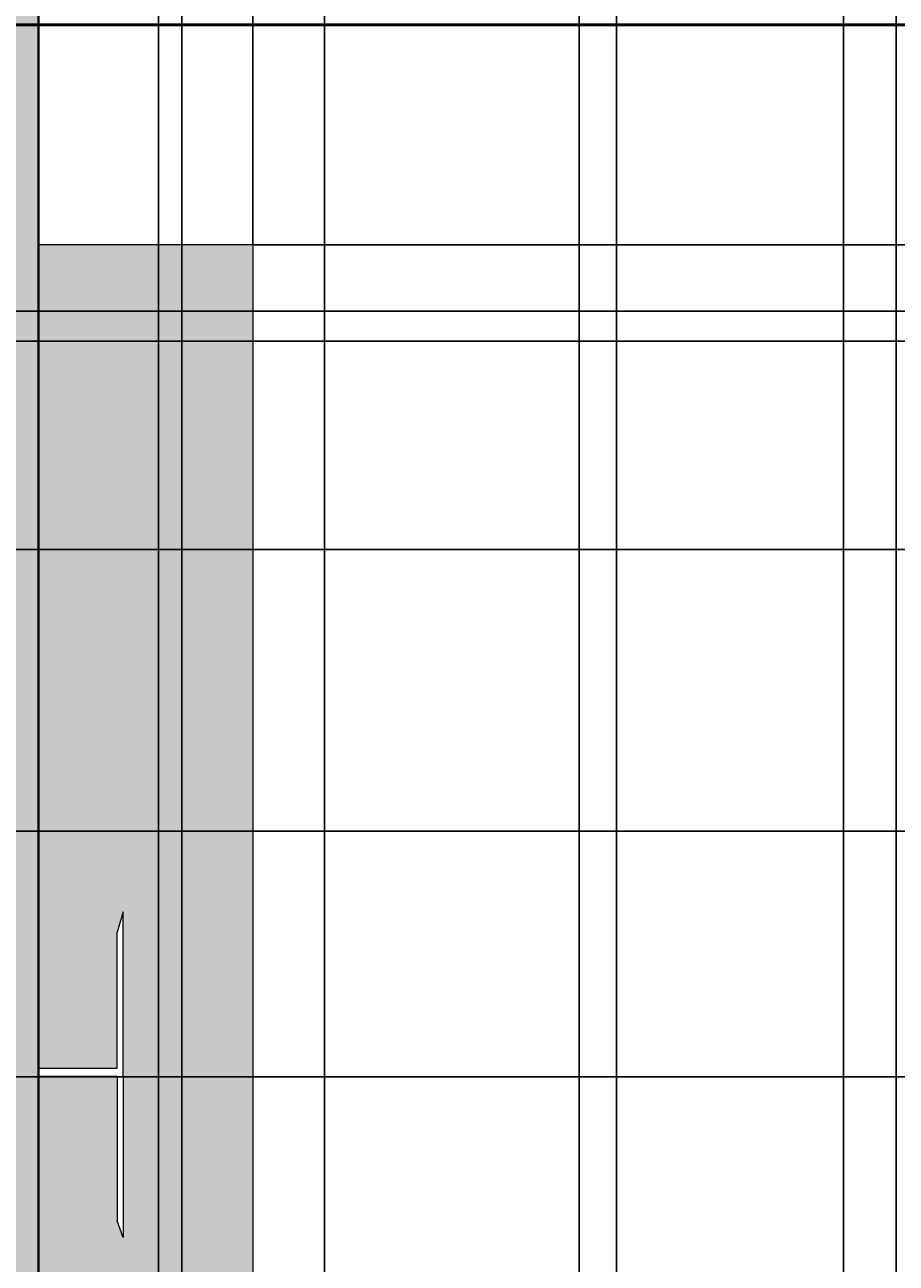
# Model space of a CAD drawing. Units: inches. Extents: x 818 to 1898, y 976 to 2364.
# Tile 26 of 96: x 1439 to 1512, y 1441 to 1545. Entities that reach past the tile are written whole.
import ezdxf

# ---------------------------------------------------------------- set-up
doc = ezdxf.new("R2010")
doc.units = ezdxf.units.IN
doc.header["$LTSCALE"] = 5
doc.header["$MEASUREMENT"] = 0
for name, color, linetype, lineweight in [('A-ANNO-DIMS', 2, 'Continuous', 18), ('A-EQPM', 8, 'Continuous', 18), ('A-FLOR-CASE', 8, 'Continuous', 18), ('A-FLOR-CASE-PATT', 33, 'Continuous', 9), ('A-WALL', 7, 'Continuous', 40)]:
    doc.layers.add(name, color=color, linetype=linetype, lineweight=lineweight)
doc.layers.add('A-WALL-PATT', color=251, linetype='Continuous', lineweight=13, true_color=0x636466)
doc.styles.get("Standard").update_dxf_attribs({"font": 'arial.ttf'})
doc.dimstyles.get("Standard").update_dxf_attribs({"dimtxt": 0.18, "dimasz": 0.18, "dimexe": 0.18, "dimexo": 0.0625, "dimgap": 0.09, "dimtad": 0, "dimtih": 1, "dimtoh": 1, "dimdec": 4, "dimzin": 0, "dimdsep": 46, "dimtxsty": 'Standard', "dimcen": 0.09, "dimadec": 0, "dimazin": 0, "dimtfac": 1, "dimtdec": 4, "dimtofl": 0, "dimtmove": 0, "dimatfit": 3, "dimfxl": 1, "dimtolj": 1, "dimtzin": 0, "dimarcsym": 0})

# ---------------------------------------------------------------- blocks, each defined once
blk = doc.blocks.new('*D99')
at = {"layer": 'A-ANNO-DIMS', "color": 0, "lineweight": -2, "ltscale": 5, "transparency": 16777216}
for p, q in [((1391.88, 1071.12), (1391.88, 2363.87)), ((1392.06, 2363.69), (1420.45, 2363.69)), ((1449.64, 2363.69), (1421.24, 2363.69)), ((1449.82, 1071.12), (1449.82, 2363.87))]:
    blk.add_line(p, q, dxfattribs=at)
at = {"layer": 'A-ANNO-DIMS', "color": 0, "ltscale": 5, "transparency": 16777216}
for points in [[(1392.06, 2363.72), (1392.06, 2363.66), (1391.88, 2363.69)], [(1449.64, 2363.72), (1449.64, 2363.66), (1449.82, 2363.69)]]:
    blk.add_solid(points, dxfattribs=at)
at = {"layer": 'Defpoints', "color": 0, "ltscale": 5, "transparency": 16777216}
for p in [(1449.82, 2363.69), (1391.88, 1071.06), (1449.82, 1071.06)]:
    blk.add_point(p, dxfattribs=at)
at = {"layer": 'A-ANNO-DIMS', "color": 0, "ltscale": 5, "transparency": 16777216, "insert": (1420.85, 2363.69), "char_height": 0.18, "attachment_point": 5}
blk.add_mtext('\\A1;57.94', dxfattribs=at)
blk = doc.blocks.new('*D100')
at = {"layer": 'A-ANNO-DIMS', "color": 0, "lineweight": -2, "ltscale": 5, "transparency": 16777216}
for p, q in [((1449.82, 1071.12), (1449.82, 2363.87)), ((1450, 2363.69), (1478.17, 2363.69)), ((1507.12, 2363.69), (1478.95, 2363.69)), ((1507.3, 1071.12), (1507.3, 2363.87))]:
    blk.add_line(p, q, dxfattribs=at)
at = {"layer": 'A-ANNO-DIMS', "color": 0, "ltscale": 5, "transparency": 16777216}
for points in [[(1450, 2363.72), (1450, 2363.66), (1449.82, 2363.69)], [(1507.12, 2363.72), (1507.12, 2363.66), (1507.3, 2363.69)]]:
    blk.add_solid(points, dxfattribs=at)
at = {"layer": 'Defpoints', "color": 0, "ltscale": 5, "transparency": 16777216}
for p in [(1507.3, 2363.69), (1449.82, 1071.06), (1507.3, 1071.06)]:
    blk.add_point(p, dxfattribs=at)
at = {"layer": 'A-ANNO-DIMS', "color": 0, "ltscale": 5, "transparency": 16777216, "insert": (1478.56, 2363.69), "char_height": 0.18, "attachment_point": 5}
blk.add_mtext('\\A1;57.48', dxfattribs=at)
blk = doc.blocks.new('*D101')
at = {"layer": 'A-ANNO-DIMS', "color": 0, "lineweight": -2, "ltscale": 5, "transparency": 16777216}
for p, q in [((1507.3, 1071.12), (1507.3, 2363.87)), ((1507.48, 2363.69), (1536, 2363.69)), ((1565.3, 2363.69), (1536.78, 2363.69)), ((1565.48, 1071.12), (1565.48, 2363.87))]:
    blk.add_line(p, q, dxfattribs=at)
at = {"layer": 'A-ANNO-DIMS', "color": 0, "ltscale": 5, "transparency": 16777216}
for points in [[(1507.48, 2363.72), (1507.48, 2363.66), (1507.3, 2363.69)], [(1565.3, 2363.72), (1565.3, 2363.66), (1565.48, 2363.69)]]:
    blk.add_solid(points, dxfattribs=at)
at = {"layer": 'Defpoints', "color": 0, "ltscale": 5, "transparency": 16777216}
for p in [(1565.48, 2363.69), (1507.3, 1071.06), (1565.48, 1071.06)]:
    blk.add_point(p, dxfattribs=at)
at = {"layer": 'A-ANNO-DIMS', "color": 0, "ltscale": 5, "transparency": 16777216, "insert": (1536.39, 2363.69), "char_height": 0.18, "attachment_point": 5}
blk.add_mtext('\\A1;58.19', dxfattribs=at)
blk = doc.blocks.new('*D116')
at = {"layer": 'A-ANNO-DIMS', "color": 0, "lineweight": -2, "ltscale": 5, "transparency": 16777216}
for p, q in [((1766.29, 1456.81), (818.03, 1456.81)), ((818.21, 1456.63), (818.21, 1417.41)), ((818.21, 1377.84), (818.21, 1417.05)), ((1766.29, 1377.66), (818.03, 1377.66))]:
    blk.add_line(p, q, dxfattribs=at)
at = {"layer": 'A-ANNO-DIMS', "color": 0, "ltscale": 5, "transparency": 16777216}
for points in [[(818.18, 1456.63), (818.24, 1456.63), (818.21, 1456.81)], [(818.18, 1377.84), (818.24, 1377.84), (818.21, 1377.66)]]:
    blk.add_solid(points, dxfattribs=at)
at = {"layer": 'Defpoints', "color": 0, "ltscale": 5, "transparency": 16777216}
for p in [(818.21, 1456.81), (1766.35, 1456.81), (1766.35, 1377.66)]:
    blk.add_point(p, dxfattribs=at)
at = {"layer": 'A-ANNO-DIMS', "color": 0, "ltscale": 5, "transparency": 16777216, "insert": (818.21, 1417.23), "char_height": 0.18, "attachment_point": 5}
blk.add_mtext('\\A1;79.15', dxfattribs=at)
blk = doc.blocks.new('*D117')
at = {"layer": 'A-ANNO-DIMS', "color": 0, "lineweight": -2, "ltscale": 5, "transparency": 16777216}
for p, q in [((1766.29, 1545.18), (818.03, 1545.18)), ((818.21, 1545), (818.21, 1501.18)), ((818.21, 1456.99), (818.21, 1500.81)), ((1766.29, 1456.81), (818.03, 1456.81))]:
    blk.add_line(p, q, dxfattribs=at)
at = {"layer": 'A-ANNO-DIMS', "color": 0, "ltscale": 5, "transparency": 16777216}
for points in [[(818.18, 1545), (818.24, 1545), (818.21, 1545.18)], [(818.18, 1456.99), (818.24, 1456.99), (818.21, 1456.81)]]:
    blk.add_solid(points, dxfattribs=at)
at = {"layer": 'Defpoints', "color": 0, "ltscale": 5, "transparency": 16777216}
for p in [(818.21, 1545.18), (1766.35, 1545.18), (1766.35, 1456.81)]:
    blk.add_point(p, dxfattribs=at)
at = {"layer": 'A-ANNO-DIMS', "color": 0, "ltscale": 5, "transparency": 16777216, "insert": (818.21, 1501), "char_height": 0.18, "attachment_point": 5}
blk.add_mtext('\\A1;88.37', dxfattribs=at)
blk = doc.blocks.new('*D159')
at = {"layer": 'A-ANNO-DIMS', "color": 0, "lineweight": -2, "ltscale": 5, "transparency": 16777216}
for p, q in [((1206.73, 1687.02), (1206.73, 975.66)), ((1463.73, 1687.02), (1463.73, 975.66)), ((1206.91, 975.84), (1334.93, 975.84)), ((1463.55, 975.84), (1335.52, 975.84))]:
    blk.add_line(p, q, dxfattribs=at)
at = {"layer": 'A-ANNO-DIMS', "color": 0, "ltscale": 5, "transparency": 16777216}
for points in [[(1206.91, 975.87), (1206.91, 975.81), (1206.73, 975.84)], [(1463.55, 975.87), (1463.55, 975.81), (1463.73, 975.84)]]:
    blk.add_solid(points, dxfattribs=at)
at = {"layer": 'Defpoints', "color": 0, "ltscale": 5, "transparency": 16777216}
for p in [(1206.73, 1687.08), (1463.73, 1687.08), (1463.73, 975.84)]:
    blk.add_point(p, dxfattribs=at)
at = {"layer": 'A-ANNO-DIMS', "color": 0, "ltscale": 5, "transparency": 16777216, "insert": (1335.23, 975.84), "char_height": 0.18, "attachment_point": 5}
blk.add_mtext('\\A1;257', dxfattribs=at)
blk = doc.blocks.new('*D160')
at = {"layer": 'A-ANNO-DIMS', "color": 0, "lineweight": -2, "ltscale": 5, "transparency": 16777216}
for p, q in [((1463.73, 1687.02), (1463.73, 975.66)), ((1511.73, 1687.02), (1511.73, 975.66)), ((1463.91, 975.84), (1487.5, 975.84)), ((1511.55, 975.84), (1487.95, 975.84))]:
    blk.add_line(p, q, dxfattribs=at)
at = {"layer": 'A-ANNO-DIMS', "color": 0, "ltscale": 5, "transparency": 16777216}
for points in [[(1463.91, 975.87), (1463.91, 975.81), (1463.73, 975.84)], [(1511.55, 975.87), (1511.55, 975.81), (1511.73, 975.84)]]:
    blk.add_solid(points, dxfattribs=at)
at = {"layer": 'Defpoints', "color": 0, "ltscale": 5, "transparency": 16777216}
for p in [(1463.73, 1687.08), (1511.73, 1687.08), (1511.73, 975.84)]:
    blk.add_point(p, dxfattribs=at)
at = {"layer": 'A-ANNO-DIMS', "color": 0, "ltscale": 5, "transparency": 16777216, "insert": (1487.73, 975.84), "char_height": 0.18, "attachment_point": 5}
blk.add_mtext('\\A1;48', dxfattribs=at)
blk = doc.blocks.new('*D170')
at = {"layer": 'A-ANNO-DIMS', "color": 0, "lineweight": -2, "ltscale": 5, "transparency": 16777216}
for p, q in [((1430.79, 1600.08), (1897.92, 1600.08)), ((1897.74, 1599.9), (1897.74, 1550.76)), ((1897.74, 1501.26), (1897.74, 1550.4)), ((1430.79, 1501.08), (1897.92, 1501.08))]:
    blk.add_line(p, q, dxfattribs=at)
at = {"layer": 'A-ANNO-DIMS', "color": 0, "ltscale": 5, "transparency": 16777216}
for points in [[(1897.71, 1599.9), (1897.77, 1599.9), (1897.74, 1600.08)], [(1897.71, 1501.26), (1897.77, 1501.26), (1897.74, 1501.08)]]:
    blk.add_solid(points, dxfattribs=at)
at = {"layer": 'Defpoints', "color": 0, "ltscale": 5, "transparency": 16777216}
for p in [(1430.73, 1600.08), (1897.74, 1600.08), (1430.73, 1501.08)]:
    blk.add_point(p, dxfattribs=at)
at = {"layer": 'A-ANNO-DIMS', "color": 0, "ltscale": 5, "transparency": 16777216, "insert": (1897.74, 1550.58), "char_height": 0.18, "attachment_point": 5}
blk.add_mtext('\\A1;99', dxfattribs=at)
blk = doc.blocks.new('*D182')
at = {"layer": 'A-ANNO-DIMS', "color": 0, "lineweight": -2, "ltscale": 5, "transparency": 16777216}
for p, q in [((1463.73, 1687.02), (1463.73, 975.66)), ((1559.73, 1687.02), (1559.73, 975.66)), ((1463.91, 975.84), (1511.51, 975.84)), ((1559.55, 975.84), (1511.94, 975.84))]:
    blk.add_line(p, q, dxfattribs=at)
at = {"layer": 'A-ANNO-DIMS', "color": 0, "ltscale": 5, "transparency": 16777216}
for points in [[(1463.91, 975.87), (1463.91, 975.81), (1463.73, 975.84)], [(1559.55, 975.87), (1559.55, 975.81), (1559.73, 975.84)]]:
    blk.add_solid(points, dxfattribs=at)
at = {"layer": 'Defpoints', "color": 0, "ltscale": 5, "transparency": 16777216}
for p in [(1463.73, 1687.08), (1559.73, 1687.08), (1559.73, 975.84)]:
    blk.add_point(p, dxfattribs=at)
at = {"layer": 'A-ANNO-DIMS', "color": 0, "ltscale": 5, "transparency": 16777216, "insert": (1511.73, 975.84), "char_height": 0.18, "attachment_point": 5}
blk.add_mtext('\\A1;96', dxfattribs=at)
blk = doc.blocks.new('*D187')
at = {"layer": 'A-ANNO-DIMS', "color": 0, "lineweight": -2, "ltscale": 5, "transparency": 16777216}
for p, q in [((1705.66, 1545.08), (818.03, 1545.08)), ((818.21, 1544.9), (818.21, 1533.26)), ((818.21, 1521.26), (818.21, 1532.9)), ((1705.66, 1521.08), (818.03, 1521.08))]:
    blk.add_line(p, q, dxfattribs=at)
at = {"layer": 'A-ANNO-DIMS', "color": 0, "ltscale": 5, "transparency": 16777216}
for points in [[(818.18, 1544.9), (818.24, 1544.9), (818.21, 1545.08)], [(818.18, 1521.26), (818.24, 1521.26), (818.21, 1521.08)]]:
    blk.add_solid(points, dxfattribs=at)
at = {"layer": 'Defpoints', "color": 0, "ltscale": 5, "transparency": 16777216}
for p in [(818.21, 1545.08), (1705.73, 1545.08), (1705.73, 1521.08)]:
    blk.add_point(p, dxfattribs=at)
at = {"layer": 'A-ANNO-DIMS', "color": 0, "ltscale": 5, "transparency": 16777216, "insert": (818.21, 1533.08), "char_height": 0.18, "attachment_point": 5}
blk.add_mtext('\\A1;24', dxfattribs=at)
blk = doc.blocks.new('*D196')
at = {"layer": 'A-ANNO-DIMS', "color": 0, "lineweight": -2, "ltscale": 5, "transparency": 16777216}
for p, q in [((1439.73, 1526.73), (1439.73, 2363.87)), ((1439.91, 2363.69), (1448.51, 2363.69)), ((1457.55, 2363.69), (1448.94, 2363.69)), ((1457.73, 1526.73), (1457.73, 2363.87))]:
    blk.add_line(p, q, dxfattribs=at)
at = {"layer": 'A-ANNO-DIMS', "color": 0, "ltscale": 5, "transparency": 16777216}
for points in [[(1439.91, 2363.72), (1439.91, 2363.66), (1439.73, 2363.69)], [(1457.55, 2363.72), (1457.55, 2363.66), (1457.73, 2363.69)]]:
    blk.add_solid(points, dxfattribs=at)
at = {"layer": 'Defpoints', "color": 0, "ltscale": 5, "transparency": 16777216}
for p in [(1457.73, 2363.69), (1439.73, 1526.67), (1457.73, 1526.67)]:
    blk.add_point(p, dxfattribs=at)
at = {"layer": 'A-ANNO-DIMS', "color": 0, "ltscale": 5, "transparency": 16777216, "insert": (1448.73, 2363.69), "char_height": 0.18, "attachment_point": 5}
blk.add_mtext('\\A1;18', dxfattribs=at)
blk = doc.blocks.new('*D197')
at = {"layer": 'A-ANNO-DIMS', "color": 0, "lineweight": -2, "ltscale": 5, "transparency": 16777216}
for p, q in [((1457.79, 1526.67), (1897.92, 1526.67)), ((1897.74, 1526.49), (1897.74, 1468.08)), ((1897.74, 1409.3), (1897.74, 1467.71)), ((1457.79, 1409.12), (1897.92, 1409.12))]:
    blk.add_line(p, q, dxfattribs=at)
at = {"layer": 'A-ANNO-DIMS', "color": 0, "ltscale": 5, "transparency": 16777216}
for points in [[(1897.71, 1526.49), (1897.77, 1526.49), (1897.74, 1526.67)], [(1897.71, 1409.3), (1897.77, 1409.3), (1897.74, 1409.12)]]:
    blk.add_solid(points, dxfattribs=at)
at = {"layer": 'Defpoints', "color": 0, "ltscale": 5, "transparency": 16777216}
for p in [(1457.73, 1526.67), (1897.74, 1526.67), (1457.73, 1409.12)]:
    blk.add_point(p, dxfattribs=at)
at = {"layer": 'A-ANNO-DIMS', "color": 0, "ltscale": 5, "transparency": 16777216, "insert": (1897.74, 1467.89), "char_height": 0.18, "attachment_point": 5}
blk.add_mtext('\\A1;117.55', dxfattribs=at)
blk = doc.blocks.new('*D198')
at = {"layer": 'A-ANNO-DIMS', "color": 0, "lineweight": -2, "ltscale": 5, "transparency": 16777216}
for p, q in [((1741.84, 1545.02), (1741.84, 975.66)), ((1430.73, 1346.02), (1430.73, 975.66)), ((1430.91, 975.84), (1585.91, 975.84)), ((1741.66, 975.84), (1586.66, 975.84))]:
    blk.add_line(p, q, dxfattribs=at)
at = {"layer": 'A-ANNO-DIMS', "color": 0, "ltscale": 5, "transparency": 16777216}
for points in [[(1430.91, 975.87), (1430.91, 975.81), (1430.73, 975.84)], [(1741.66, 975.87), (1741.66, 975.81), (1741.84, 975.84)]]:
    blk.add_solid(points, dxfattribs=at)
at = {"layer": 'Defpoints', "color": 0, "ltscale": 5, "transparency": 16777216}
for p in [(1741.84, 1545.08), (1430.73, 1346.08), (1741.84, 975.84)]:
    blk.add_point(p, dxfattribs=at)
at = {"layer": 'A-ANNO-DIMS', "color": 0, "ltscale": 5, "transparency": 16777216, "insert": (1586.28, 975.84), "char_height": 0.18, "attachment_point": 5}
blk.add_mtext('\\A1;311.1', dxfattribs=at)
blk = doc.blocks.new('*D201')
at = {"layer": 'A-ANNO-DIMS', "color": 0, "lineweight": -2, "ltscale": 5, "transparency": 16777216}
for p, q in [((1678.27, 1518.56), (818.03, 1518.56)), ((818.21, 1518.38), (818.21, 1498.18)), ((818.21, 1477.61), (818.21, 1497.81)), ((1678.27, 1477.43), (818.03, 1477.43))]:
    blk.add_line(p, q, dxfattribs=at)
at = {"layer": 'A-ANNO-DIMS', "color": 0, "ltscale": 5, "transparency": 16777216}
for points in [[(818.18, 1518.38), (818.24, 1518.38), (818.21, 1518.56)], [(818.18, 1477.61), (818.24, 1477.61), (818.21, 1477.43)]]:
    blk.add_solid(points, dxfattribs=at)
at = {"layer": 'Defpoints', "color": 0, "ltscale": 5, "transparency": 16777216}
for p in [(818.21, 1518.56), (1678.33, 1518.56), (1678.33, 1477.43)]:
    blk.add_point(p, dxfattribs=at)
at = {"layer": 'A-ANNO-DIMS', "color": 0, "ltscale": 5, "transparency": 16777216, "insert": (818.21, 1497.99), "char_height": 0.18, "attachment_point": 5}
blk.add_mtext('\\A1;41.135', dxfattribs=at)
blk = doc.blocks.new('*D214')
at = {"layer": 'A-ANNO-DIMS', "color": 0, "lineweight": -2, "ltscale": 5, "transparency": 16777216}
for p, q in [((1511.73, 1687.02), (1511.73, 975.66)), ((1714.73, 1687.02), (1714.73, 975.66)), ((1511.91, 975.84), (1612.93, 975.84)), ((1714.55, 975.84), (1613.52, 975.84))]:
    blk.add_line(p, q, dxfattribs=at)
at = {"layer": 'A-ANNO-DIMS', "color": 0, "ltscale": 5, "transparency": 16777216}
for points in [[(1511.91, 975.87), (1511.91, 975.81), (1511.73, 975.84)], [(1714.55, 975.87), (1714.55, 975.81), (1714.73, 975.84)]]:
    blk.add_solid(points, dxfattribs=at)
at = {"layer": 'Defpoints', "color": 0, "ltscale": 5, "transparency": 16777216}
for p in [(1511.73, 1687.08), (1714.73, 1687.08), (1714.73, 975.84)]:
    blk.add_point(p, dxfattribs=at)
at = {"layer": 'A-ANNO-DIMS', "color": 0, "ltscale": 5, "transparency": 16777216, "insert": (1613.23, 975.84), "char_height": 0.18, "attachment_point": 5}
blk.add_mtext('\\A1;203', dxfattribs=at)
blk = doc.blocks.new('*D242')
at = {"layer": 'A-ANNO-DIMS', "color": 0, "lineweight": -2, "ltscale": 5, "transparency": 16777216}
for p, q in [((1488.26, 1948.6), (1488.26, 975.66)), ((1513.23, 1948.6), (1513.23, 975.66)), ((1488.44, 975.84), (1500.35, 975.84)), ((1513.05, 975.84), (1501.14, 975.84))]:
    blk.add_line(p, q, dxfattribs=at)
at = {"layer": 'A-ANNO-DIMS', "color": 0, "ltscale": 5, "transparency": 16777216}
for points in [[(1488.44, 975.87), (1488.44, 975.81), (1488.26, 975.84)], [(1513.05, 975.87), (1513.05, 975.81), (1513.23, 975.84)]]:
    blk.add_solid(points, dxfattribs=at)
at = {"layer": 'Defpoints', "color": 0, "ltscale": 5, "transparency": 16777216}
for p in [(1488.26, 1948.66), (1513.23, 1948.66), (1513.23, 975.84)]:
    blk.add_point(p, dxfattribs=at)
at = {"layer": 'A-ANNO-DIMS', "color": 0, "ltscale": 5, "transparency": 16777216, "insert": (1500.74, 975.84), "char_height": 0.18, "attachment_point": 5}
blk.add_mtext('\\A1;24.97', dxfattribs=at)
blk = doc.blocks.new('*D243')
at = {"layer": 'A-ANNO-DIMS', "color": 0, "lineweight": -2, "ltscale": 5, "transparency": 16777216}
for p, q in [((1451.77, 2020.02), (1451.77, 975.66)), ((1590.73, 2020.02), (1590.73, 975.66)), ((1451.95, 975.84), (1520.79, 975.84)), ((1590.55, 975.84), (1521.7, 975.84))]:
    blk.add_line(p, q, dxfattribs=at)
at = {"layer": 'A-ANNO-DIMS', "color": 0, "ltscale": 5, "transparency": 16777216}
for points in [[(1451.95, 975.87), (1451.95, 975.81), (1451.77, 975.84)], [(1590.55, 975.87), (1590.55, 975.81), (1590.73, 975.84)]]:
    blk.add_solid(points, dxfattribs=at)
at = {"layer": 'Defpoints', "color": 0, "ltscale": 5, "transparency": 16777216}
for p in [(1451.77, 2020.08), (1590.73, 2020.08), (1590.73, 975.84)]:
    blk.add_point(p, dxfattribs=at)
at = {"layer": 'A-ANNO-DIMS', "color": 0, "ltscale": 5, "transparency": 16777216, "insert": (1521.25, 975.84), "char_height": 0.18, "attachment_point": 5}
blk.add_mtext('\\A1;138.96', dxfattribs=at)
blk = doc.blocks.new('*D253')
at = {"layer": 'A-ANNO-DIMS', "color": 0, "lineweight": -2, "ltscale": 5, "transparency": 16777216}
for p, q in [((1485.12, 2053.02), (1485.12, 975.66)), ((1538.52, 2053.02), (1538.52, 975.66)), ((1485.3, 975.84), (1511.42, 975.84)), ((1538.34, 975.84), (1512.21, 975.84))]:
    blk.add_line(p, q, dxfattribs=at)
at = {"layer": 'A-ANNO-DIMS', "color": 0, "ltscale": 5, "transparency": 16777216}
for points in [[(1485.3, 975.87), (1485.3, 975.81), (1485.12, 975.84)], [(1538.34, 975.87), (1538.34, 975.81), (1538.52, 975.84)]]:
    blk.add_solid(points, dxfattribs=at)
at = {"layer": 'Defpoints', "color": 0, "ltscale": 5, "transparency": 16777216}
for p in [(1485.12, 2053.08), (1538.52, 2053.08), (1538.52, 975.84)]:
    blk.add_point(p, dxfattribs=at)
at = {"layer": 'A-ANNO-DIMS', "color": 0, "ltscale": 5, "transparency": 16777216, "insert": (1511.82, 975.84), "char_height": 0.18, "attachment_point": 5}
blk.add_mtext('\\A1;53.39', dxfattribs=at)

msp = doc.modelspace()

# ---------------------------------------------------------------- hatches: boundary and pattern name
at = {"layer": 'A-FLOR-CASE-PATT', "ltscale": 5}
h = msp.add_hatch(color=256, dxfattribs=at)
h.dxf.hatch_style = 1
h.paths.add_polyline_path([(1705.7251, 1941.0782), (1681.7252, 1941.0782), (1681.7252, 1900.0782), (1599.7252, 1900.0782), (1599.7252, 1876.0782), (1705.7251, 1876.0782)])
h.paths.add_polyline_path([(1457.7251, 1409.1177), (1457.7251, 1526.6712), (1439.7251, 1526.6712), (1439.7251, 1457.5313), (1446.3307, 1457.5313), (1446.3307, 1468.9514), (1446.8307, 1470.665), (1446.8307, 1469.665), (1446.8307, 1468.9514), (1446.8307, 1456.8361), (1446.8307, 1444.7258), (1446.8307, 1443.3338), (1446.3307, 1444.7258), (1446.3307, 1456.8361), (1439.7251, 1456.8361), (1439.7251, 1355.0782), (1463.7251, 1355.0782), (1463.7251, 1367.3287), (1458.0475, 1367.3287, -0.23606798), (1457.0475, 1369.3287), (1456.0475, 1369.3287, -0.11764706), (1456.0475, 1386.3287), (1457.0475, 1386.3287, -0.23606798), (1458.0475, 1388.3287), (1463.7251, 1388.3287), (1463.7251, 1389.3211)])
h.paths.add_polyline_path([(1341.2593, 1534.0782), (1246.9377, 1534.0782), (1246.9377, 1510.0782), (1341.2593, 1510.0782)])
h.paths.add_polyline_path([(1288.8272, 1519.927), (1289.8272, 1519.927), (1290.5408, 1519.927), (1302.6561, 1519.927), (1314.7664, 1519.927), (1316.1584, 1519.927), (1314.7664, 1519.427), (1302.6561, 1519.427), (1302.6561, 1512.8214), (1301.9609, 1512.8214), (1301.9609, 1519.427), (1290.5408, 1519.427)], flags=16)
h.paths.add_polyline_path([(1377.7791, 1867.0782), (1344.5531, 1867.0782), (1344.5531, 1860.4726), (1355.9731, 1860.4726), (1357.6867, 1859.9726), (1356.6867, 1859.9726), (1355.9731, 1859.9726), (1343.8579, 1859.9726), (1331.7475, 1859.9726), (1330.3556, 1859.9726), (1331.7475, 1860.4726), (1343.8579, 1860.4726), (1343.8579, 1867.0782), (1311.3271, 1867.0782), (1311.3271, 1853.7496), (1377.7791, 1853.7496)])
h.paths.add_polyline_path([(1301.148, 1610.7299, -0.46196039), (1314.4882, 1599.3725, -0.19222541), (1311.3254, 1591.4497, 0.54791519), (1336.8832, 1607.7707, 0.92061359)])
h.paths.add_polyline_path([(1370.719, 1780.5695, 1), (1332.478, 1780.5695, 1)])
h.paths.add_polyline_path([(1705.7251, 1463.0782), (1681.7252, 1463.0782), (1681.7252, 1379.0782), (1622.7252, 1379.0782), (1622.7252, 1355.0782), (1705.7251, 1355.0782)])
h.paths.add_polyline_path([(1658.1052, 1359.2188), (1658.1786, 1359.2188), (1658.1786, 1373.8763), (1658.1052, 1373.9202)], flags=16)
h.paths.add_polyline_path([(1686.9271, 1409.9311), (1686.8832, 1409.8578), (1701.5845, 1409.8578), (1701.5845, 1409.9311)], flags=16)
h.paths.add_polyline_path([(1637.1266, 1359.2188), (1637.2, 1359.2188), (1637.2, 1373.8763), (1637.1266, 1373.9202)], flags=16)
at = {"layer": 'A-WALL-PATT', "ltscale": 5}
h = msp.add_hatch(color=256, dxfattribs=at)
h.dxf.hatch_style = 1
h.paths.add_polyline_path([(1206.7251, 1687.0782), (1206.7251, 1700.0782), (1197.7252, 1700.0782), (1197.7252, 1501.0782), (1206.7251, 1501.0782), (1206.7251, 1510.0782)])
h.paths.add_polyline_path([(1197.7252, 1590.7585), (1173.7252, 1590.7585), (1173.7252, 1586.7585), (1197.7252, 1586.7585)])
h.paths.add_polyline_path([(1197.7252, 1534.6024), (1173.7252, 1534.6024), (1173.7252, 1530.6024), (1197.7252, 1530.6024)])
h.paths.add_polyline_path([(1365.1463, 1510.0782), (1283.8183, 1510.0782), (1283.8183, 1501.0782), (1365.1463, 1501.0782)])
h.paths.add_polyline_path([(1439.7251, 1591.0782), (1441.7252, 1591.0782), (1441.7252, 1600.0782), (1430.7251, 1600.0782), (1430.7251, 1510.0782), (1406.7252, 1510.0782), (1401.1463, 1510.0782), (1401.1463, 1501.0782), (1430.7251, 1501.0782), (1430.7251, 1486.2383), (1430.7251, 1409.0522), (1439.7251, 1409.0522)])

# ---------------------------------------------------------------- linework, layer by layer
at = {"layer": 'A-EQPM'}
for p, q in [((1446.8307, 1470.665), (1446.3307, 1468.9514)), ((1446.8307, 1469.665), (1446.8307, 1470.665)), ((1446.8307, 1468.9514), (1446.8307, 1469.665)), ((1446.3307, 1457.5313), (1446.3307, 1468.9514)), ((1446.8307, 1456.8361), (1446.8307, 1468.9514)), ((1446.3307, 1456.8361), (1446.3307, 1444.7258)), ((1446.8307, 1456.8361), (1446.8307, 1444.7258)), ((1446.8307, 1443.3338), (1446.3307, 1444.7258)), ((1446.8307, 1444.7258), (1446.8307, 1443.3338))]:
    msp.add_line(p, q, dxfattribs=at)
msp.add_lwpolyline([(1446.3307, 1456.8361), (1439.7251, 1456.8361), (1439.7251, 1457.5313), (1446.3307, 1457.5313)], dxfattribs=at)
at = {"layer": 'A-FLOR-CASE'}
for p, q in [((1439.7251, 1526.6712), (1457.7251, 1526.6712)), ((1457.7251, 1526.6712), (1457.7251, 1409.1177))]:
    msp.add_line(p, q, dxfattribs=at)
at = {"layer": 'A-WALL'}
msp.add_line((1439.7251, 1591.0782), (1439.7251, 1355.0782), dxfattribs=at)

# ---------------------------------------------------------------- dimensions: what is measured, and where the dimension line sits
at = {"layer": 'A-ANNO-DIMS', "ltscale": 5}
for base, p1, p2, override, picture, middle in [((1449.8196, 2363.6929), (1391.8757, 1071.0552), (1449.8196, 1071.0552), {"dimdec": 2, "dimlfac": 1, "dimrnd": 0, "dimzin": 0, "dimdsep": 46, "dimlunit": 2}, '*D99', (1420.8477, 2363.6929)), ((1457.7251, 2363.6929), (1439.7251, 1526.6712), (1457.7251, 1526.6712), {"dimdec": 0, "dimlfac": 1, "dimrnd": 0, "dimzin": 0, "dimdsep": 46, "dimlunit": 2}, '*D196', (1448.7251, 2363.6929)), ((1507.2982, 2363.6929), (1449.8196, 1071.0552), (1507.2982, 1071.0552), {"dimdec": 2, "dimlfac": 1, "dimrnd": 0, "dimzin": 0, "dimdsep": 46, "dimlunit": 2}, '*D100', (1478.5589, 2363.6929)), ((1565.4835, 2363.6929), (1507.2982, 1071.0552), (1565.4835, 1071.0552), {"dimdec": 2, "dimlfac": 1, "dimrnd": 0, "dimzin": 0, "dimdsep": 46, "dimlunit": 2}, '*D101', (1536.3908, 2363.6929)), ((1538.5155, 975.8433), (1485.1216, 2053.0782), (1538.5155, 2053.0782), {"dimdec": 2, "dimlfac": 1, "dimrnd": 0, "dimzin": 0, "dimdsep": 46, "dimlunit": 2}, '*D253', (1511.8185, 975.8433)), ((1590.7251, 975.8433), (1451.7698, 2020.0782), (1590.7251, 2020.0782), {"dimdec": 2, "dimlfac": 1, "dimrnd": 0, "dimzin": 0, "dimdsep": 46, "dimlunit": 2}, '*D243', (1521.2475, 975.8433)), ((1513.2306, 975.8433), (1488.2586, 1948.6602), (1513.2306, 1948.6602), {"dimdec": 2, "dimlfac": 1, "dimrnd": 0, "dimzin": 0, "dimdsep": 46, "dimlunit": 2}, '*D242', (1500.7446, 975.8433)), ((1463.7251, 975.8433), (1206.7251, 1687.0782), (1463.7251, 1687.0782), {"dimdec": 0, "dimlfac": 1, "dimrnd": 0, "dimzin": 0, "dimdsep": 46, "dimlunit": 2}, '*D159', (1335.2251, 975.8433)), ((1511.7251, 975.8433), (1463.7251, 1687.0782), (1511.7251, 1687.0782), {"dimdec": 0, "dimlfac": 1, "dimrnd": 0, "dimzin": 0, "dimdsep": 46, "dimlunit": 2}, '*D160', (1487.7251, 975.8433)), ((1559.7251, 975.8433), (1463.7251, 1687.0782), (1559.7251, 1687.0782), {"dimdec": 0, "dimlfac": 1, "dimrnd": 0, "dimzin": 0, "dimdsep": 46, "dimlunit": 2}, '*D182', (1511.7251, 975.8433)), ((1714.7251, 975.8433), (1511.7251, 1687.0782), (1714.7251, 1687.0782), {"dimdec": 0, "dimlfac": 1, "dimrnd": 0, "dimzin": 0, "dimdsep": 46, "dimlunit": 2}, '*D214', (1613.2251, 975.8433)), ((1741.8409, 975.8433), (1430.7251, 1346.0782), (1741.8409, 1545.0782), {"dimdec": 1, "dimlfac": 1, "dimrnd": 0, "dimzin": 0, "dimdsep": 46, "dimlunit": 2}, '*D198', (1586.283, 975.8433))]:
    dim = msp.add_linear_dim(base=base, p1=p1, p2=p2, dimstyle='Standard', override=override, dxfattribs=at)
    dim.commit()
    dim.dimension.update_dxf_attribs({"geometry": picture, "text_midpoint": middle})
for base, p1, p2, override, picture, middle in [((1897.736, 1600.0782), (1430.7251, 1501.0782), (1430.7251, 1600.0782), {"dimdec": 0, "dimlfac": 1, "dimrnd": 0, "dimzin": 0, "dimdsep": 46, "dimlunit": 2}, '*D170', (1897.736, 1550.5782)), ((818.2059, 1545.1827), (1766.3524, 1456.8088), (1766.3524, 1545.1827), {"dimdec": 2, "dimlfac": 1, "dimrnd": 0, "dimzin": 0, "dimdsep": 46, "dimlunit": 2}, '*D117', (818.2059, 1500.9957)), ((818.2059, 1545.0782), (1705.7251, 1521.0782), (1705.7251, 1545.0782), {"dimdec": 0, "dimlfac": 1, "dimrnd": 0, "dimzin": 0, "dimdsep": 46, "dimlunit": 2}, '*D187', (818.2059, 1533.0782)), ((1897.736, 1526.6712), (1457.7251, 1409.1177), (1457.7251, 1526.6712), {"dimdec": 2, "dimlfac": 1, "dimrnd": 0, "dimzin": 0, "dimdsep": 46, "dimlunit": 2}, '*D197', (1897.736, 1467.8945)), ((818.2059, 1518.5611), (1678.3302, 1477.4261), (1678.3302, 1518.5611), {"dimdec": 3, "dimlfac": 1, "dimrnd": 0, "dimzin": 0, "dimdsep": 46, "dimlunit": 2}, '*D201', (818.2059, 1497.9936)), ((818.2059, 1456.8088), (1766.3524, 1377.6564), (1766.3524, 1456.8088), {"dimdec": 2, "dimlfac": 1, "dimrnd": 0, "dimzin": 0, "dimdsep": 46, "dimlunit": 2}, '*D116', (818.2059, 1417.2326))]:
    dim = msp.add_linear_dim(base=base, p1=p1, p2=p2, angle=90, dimstyle='Standard', override=override, dxfattribs=at)
    dim.commit()
    dim.dimension.update_dxf_attribs({"geometry": picture, "text_midpoint": middle})

doc.saveas('drawing.dxf')
